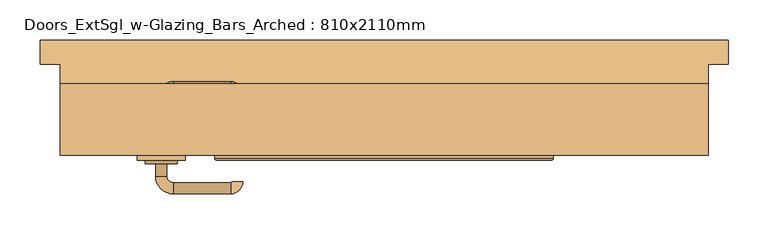
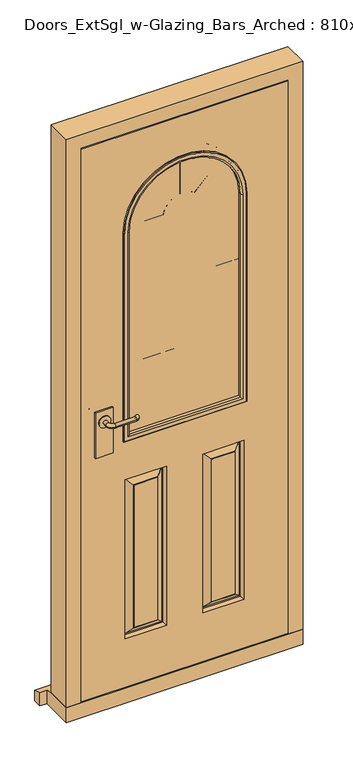
"""IFC4 building model written with IfcOpenShell, lengths in millimetres: door geometry, Doors_ExtSgl_w-Glazing_Bars_Arched : 810x2110mm."""

from ifc_helpers import new_model, si_unit, point, frame, frame_2d, origin, place, context, project, spatial, polyline, circle_curve, ellipse_curve, trimmed, segment, composite_curve, outline, extrude, faceted_brep, source, transform, mapped, element, save
from ifc_brep_helpers import plane_surface, cylinder_surface, revolved_surface, advanced_brep


def doors_extsgl_w_glazing_bars_arched_810x2110mm_57ea6d9e(model_context):
    return source(origin(), model_context, "Body", "SolidModel", [
        extrude(outline(composite_curve([segment(trimmed(circle_curve(frame_2d((1050.0, -278.5)), 20.0), [point((1050.0, -298.5))], [point((1050.0, -258.5))], False, "CARTESIAN"), True, "CONTINUOUS"), segment(trimmed(circle_curve(frame_2d((1050.0, -278.5)), 20.0), [point((1050.0, -258.5))], [point((1050.0, -298.5))], False, "CARTESIAN"), True, "CONTINUOUS")], self_intersect=False)), frame((0.0, -22.9929895, 0.0), z_axis=(0.0, 1.0, 0.0), x_axis=(0.0, 0.0, 1.0)), (0.0, 0.0, 1.0), 4.5929895),
        advanced_brep(
        [(-271.5, -22.9929895, 1050.0), (-285.5, -22.9929895, 1050.0), (-285.5, -38.4, 1050.0), (-271.5, -38.4, 1050.0), (-263.5, -60.4, 1050.0), (-263.5, -46.4, 1050.0), (-191.5, -60.4, 1050.0), (-191.5, -46.4, 1050.0), (-190.5, -45.4, 1050.0), (-176.5, -45.4, 1050.0)],
        [
            (0, 1, circle_curve(frame((-278.5, -22.9929895, 1050.0), z_axis=(0.0, 1.0, 0.0), x_axis=(-1.0, 0.0, 0.0)), 7.0)),
            (1, 0, circle_curve(frame((-278.5, -22.9929895, 1050.0), z_axis=(0.0, 1.0, 0.0), x_axis=(-1.0, 0.0, 0.0)), 7.0)),
            (1, 2),
            (2, 3, circle_curve(frame((-278.5, -38.4, 1050.0), z_axis=(0.0, 1.0, 0.0), x_axis=(-1.0, 0.0, 0.0)), 7.0)),
            (3, 0),
            (3, 2, circle_curve(frame((-278.5, -38.4, 1050.0), z_axis=(0.0, 1.0, 0.0), x_axis=(-1.0, 0.0, 0.0)), 7.0)),
            (4, 5, circle_curve(frame((-263.5, -53.4, 1050.0), z_axis=(-1.0, 0.0, 0.0), x_axis=(0.0, -1.0, 0.0)), 7.0)),
            (5, 3, circle_curve(frame((-263.5, -38.4, 1050.0), z_axis=(0.0, 0.0, -1.0), x_axis=(-1.0, 0.0, 0.0)), 8.0)),
            (2, 4, circle_curve(frame((-263.5, -38.4, 1050.0), z_axis=(0.0, 0.0, 1.0), x_axis=(-1.0, 0.0, 0.0)), 22.0)),
            (5, 4, circle_curve(frame((-263.5, -53.4, 1050.0), z_axis=(-1.0, 0.0, 0.0), x_axis=(0.0, -1.0, 0.0)), 7.0)),
            (4, 6),
            (6, 7, circle_curve(frame((-191.5, -53.4, 1050.0), z_axis=(-1.0, 0.0, 0.0), x_axis=(0.0, -1.0, 0.0)), 7.0)),
            (7, 5),
            (7, 6, circle_curve(frame((-191.5, -53.4, 1050.0), z_axis=(-1.0, 0.0, 0.0), x_axis=(0.0, -1.0, 0.0)), 7.0)),
            (8, 9, circle_curve(frame((-183.5, -45.4, 1050.0), z_axis=(0.0, 1.0, 0.0), x_axis=(1.0, 0.0, 0.0)), 7.0)),
            (9, 8, circle_curve(frame((-183.5, -45.4, 1050.0), z_axis=(0.0, 1.0, 0.0), x_axis=(1.0, 0.0, 0.0)), 7.0)),
            (8, 7, circle_curve(frame((-191.5, -45.4, 1050.0), z_axis=(0.0, 0.0, -1.0), x_axis=(0.0, -1.0, 0.0)), 1.0)),
            (6, 9, circle_curve(frame((-191.5, -45.4, 1050.0), z_axis=(0.0, 0.0, 1.0), x_axis=(0.0, -1.0, 0.0)), 15.0)),
        ],
        [
            plane_surface(frame((-278.5, -22.9929895, 1050.0), z_axis=(0.0, 1.0, 0.0), x_axis=(0.0, 0.0, 1.0))),
            cylinder_surface(frame((-278.5, -22.9929895, 1050.0), z_axis=(0.0, 1.0, 0.0), x_axis=(-1.0, 0.0, 0.0)), 7.0),
            revolved_surface(trimmed(ellipse_curve(frame((-278.5, -38.4, 1050.0), z_axis=(0.0, -1.0, 0.0), x_axis=(-1.0, 0.0, 0.0)), 7.0, 7.0), [point((-271.5, -38.4, 1050.0))], [point((-285.5, -38.4, 1050.0))], True, "CARTESIAN"), (-263.5, -38.4, 1050.0), (0.0, 0.0, -1.0)),
            revolved_surface(trimmed(ellipse_curve(frame((-278.5, -38.4, 1050.0), z_axis=(0.0, -1.0, 0.0), x_axis=(-1.0, 0.0, 0.0)), 7.0, 7.0), [point((-285.5, -38.4, 1050.0))], [point((-271.5, -38.4, 1050.0))], True, "CARTESIAN"), (-263.5, -38.4, 1050.0), (0.0, 0.0, -1.0)),
            cylinder_surface(frame((-263.5, -53.4, 1050.0), z_axis=(-1.0, 0.0, 0.0), x_axis=(0.0, -1.0, 0.0)), 7.0),
            plane_surface(frame((-183.5, -45.4, 1050.0), z_axis=(0.0, 1.0, 0.0), x_axis=(0.0, 0.0, 1.0))),
            revolved_surface(trimmed(ellipse_curve(frame((-191.5, -53.4, 1050.0), z_axis=(1.0, 0.0, 0.0), x_axis=(0.0, -1.0, 0.0)), 7.0, 7.0), [point((-191.5, -46.4, 1050.0))], [point((-191.5, -60.4, 1050.0))], True, "CARTESIAN"), (-191.5, -45.4, 1050.0), (0.0, 0.0, -1.0)),
            revolved_surface(trimmed(ellipse_curve(frame((-191.5, -53.4, 1050.0), z_axis=(1.0, 0.0, 0.0), x_axis=(0.0, -1.0, 0.0)), 7.0, 7.0), [point((-191.5, -60.4, 1050.0))], [point((-191.5, -46.4, 1050.0))], True, "CARTESIAN"), (-191.5, -45.4, 1050.0), (0.0, 0.0, -1.0)),
        ],
        [
            (0, [[1, 2]]),
            (1, [[3, 4, 5, -2]]),
            (1, [[-5, 6, -3, -1]]),
            (2, [[7, 8, -4, 9]]),
            (3, [[10, -9, -6, -8]]),
            (4, [[11, 12, 13, -7]]),
            (4, [[-13, 14, -11, -10]]),
            (5, [[15, 16]]),
            (6, [[-15, 17, -12, 18]]),
            (7, [[-16, -18, -14, -17]]),
        ],
    ),
        extrude(outline(polyline([(-248.5, -12.4), (-248.5, -18.4), (-308.5, -18.4), (-308.5, -12.4), (-248.5, -12.4)])), frame((0.0, 0.0, 925.0), z_axis=(0.0, 0.0, 1.0), x_axis=(1.0, 0.0, 0.0)), (0.0, 0.0, 1.0), 165.0),
        extrude(outline(composite_curve([segment(trimmed(circle_curve(frame_2d((1050.0, -278.5)), 20.0), [point((1050.0, -298.5))], [point((1050.0, -258.5))], False, "CARTESIAN"), True, "CONTINUOUS"), segment(trimmed(circle_curve(frame_2d((1050.0, -278.5)), 20.0), [point((1050.0, -258.5))], [point((1050.0, -298.5))], False, "CARTESIAN"), True, "CONTINUOUS")], self_intersect=False)), frame((0.0, 37.6, 0.0), z_axis=(0.0, 1.0, 0.0), x_axis=(0.0, 0.0, 1.0)), (0.0, 0.0, 1.0), 4.5929895),
        advanced_brep(
        [(-271.5, 42.1929895, 1050.0), (-285.5, 42.1929895, 1050.0), (-271.5, 57.6, 1050.0), (-285.5, 57.6, 1050.0), (-263.5, 79.6, 1050.0), (-263.5, 65.6, 1050.0), (-191.5, 65.6, 1050.0), (-191.5, 79.6, 1050.0), (-190.5, 64.6, 1050.0), (-176.5, 64.6, 1050.0)],
        [
            (0, 1, circle_curve(frame((-278.5, 42.1929895, 1050.0), z_axis=(0.0, -1.0, 0.0), x_axis=(-1.0, 0.0, 0.0)), 7.0)),
            (1, 0, circle_curve(frame((-278.5, 42.1929895, 1050.0), z_axis=(0.0, -1.0, 0.0), x_axis=(-1.0, 0.0, 0.0)), 7.0)),
            (0, 2),
            (2, 3, circle_curve(frame((-278.5, 57.6, 1050.0), z_axis=(0.0, -1.0, 0.0), x_axis=(-1.0, 0.0, 0.0)), 7.0)),
            (3, 1),
            (3, 2, circle_curve(frame((-278.5, 57.6, 1050.0), z_axis=(0.0, -1.0, 0.0), x_axis=(-1.0, 0.0, 0.0)), 7.0)),
            (4, 3, circle_curve(frame((-263.5, 57.6, 1050.0), z_axis=(0.0, 0.0, 1.0), x_axis=(-1.0, 0.0, 0.0)), 22.0)),
            (2, 5, circle_curve(frame((-263.5, 57.6, 1050.0), z_axis=(0.0, 0.0, -1.0), x_axis=(-1.0, 0.0, 0.0)), 8.0)),
            (5, 4, circle_curve(frame((-263.5, 72.6, 1050.0), z_axis=(-1.0, 0.0, 0.0), x_axis=(0.0, 1.0, 0.0)), 7.0)),
            (4, 5, circle_curve(frame((-263.5, 72.6, 1050.0), z_axis=(-1.0, 0.0, 0.0), x_axis=(0.0, 1.0, 0.0)), 7.0)),
            (5, 6),
            (6, 7, circle_curve(frame((-191.5, 72.6, 1050.0), z_axis=(-1.0, 0.0, 0.0), x_axis=(0.0, 1.0, 0.0)), 7.0)),
            (7, 4),
            (7, 6, circle_curve(frame((-191.5, 72.6, 1050.0), z_axis=(-1.0, 0.0, 0.0), x_axis=(0.0, 1.0, 0.0)), 7.0)),
            (8, 9, circle_curve(frame((-183.5, 64.6, 1050.0), z_axis=(0.0, -1.0, 0.0), x_axis=(1.0, 0.0, 0.0)), 7.0)),
            (9, 8, circle_curve(frame((-183.5, 64.6, 1050.0), z_axis=(0.0, -1.0, 0.0), x_axis=(1.0, 0.0, 0.0)), 7.0)),
            (9, 7, circle_curve(frame((-191.5, 64.6, 1050.0), z_axis=(0.0, 0.0, 1.0), x_axis=(0.0, 1.0, 0.0)), 15.0)),
            (6, 8, circle_curve(frame((-191.5, 64.6, 1050.0), z_axis=(0.0, 0.0, -1.0), x_axis=(0.0, 1.0, 0.0)), 1.0)),
        ],
        [
            plane_surface(frame((-278.5, 42.1929895, 1050.0), z_axis=(0.0, -1.0, 0.0), x_axis=(0.0, 0.0, 1.0))),
            cylinder_surface(frame((-278.5, 42.1929895, 1050.0), z_axis=(0.0, -1.0, 0.0), x_axis=(-1.0, 0.0, 0.0)), 7.0),
            revolved_surface(trimmed(ellipse_curve(frame((-278.5, 57.6, 1050.0), z_axis=(0.0, -1.0, 0.0), x_axis=(-1.0, 0.0, 0.0)), 7.0, 7.0), [point((-271.5, 57.6, 1050.0))], [point((-285.5, 57.6, 1050.0))], True, "CARTESIAN"), (-263.5, 57.6, 1050.0), (0.0, 0.0, -1.0)),
            revolved_surface(trimmed(ellipse_curve(frame((-278.5, 57.6, 1050.0), z_axis=(0.0, -1.0, 0.0), x_axis=(-1.0, 0.0, 0.0)), 7.0, 7.0), [point((-285.5, 57.6, 1050.0))], [point((-271.5, 57.6, 1050.0))], True, "CARTESIAN"), (-263.5, 57.6, 1050.0), (0.0, 0.0, -1.0)),
            cylinder_surface(frame((-263.5, 72.6, 1050.0), z_axis=(-1.0, 0.0, 0.0), x_axis=(0.0, 1.0, 0.0)), 7.0),
            plane_surface(frame((-183.5, 64.6, 1050.0), z_axis=(0.0, -1.0, 0.0), x_axis=(0.0, 0.0, 1.0))),
            revolved_surface(trimmed(ellipse_curve(frame((-191.5, 72.6, 1050.0), z_axis=(-1.0, 0.0, 0.0), x_axis=(0.0, 1.0, 0.0)), 7.0, 7.0), [point((-191.5, 65.6, 1050.0))], [point((-191.5, 79.6, 1050.0))], True, "CARTESIAN"), (-191.5, 64.6, 1050.0), (0.0, 0.0, -1.0)),
            revolved_surface(trimmed(ellipse_curve(frame((-191.5, 72.6, 1050.0), z_axis=(-1.0, 0.0, 0.0), x_axis=(0.0, 1.0, 0.0)), 7.0, 7.0), [point((-191.5, 79.6, 1050.0))], [point((-191.5, 65.6, 1050.0))], True, "CARTESIAN"), (-191.5, 64.6, 1050.0), (0.0, 0.0, -1.0)),
        ],
        [
            (0, [[1, 2]]),
            (1, [[-1, 3, 4, 5]]),
            (1, [[-2, -5, 6, -3]]),
            (2, [[7, -4, 8, 9]]),
            (3, [[-8, -6, -7, 10]]),
            (4, [[-9, 11, 12, 13]]),
            (4, [[-10, -13, 14, -11]]),
            (5, [[15, 16]]),
            (6, [[17, -12, 18, -16]]),
            (7, [[-18, -14, -17, -15]]),
        ],
    ),
        extrude(outline(polyline([(-248.5, 31.6), (-308.5, 31.6), (-308.5, 37.6), (-248.5, 37.6), (-248.5, 31.6)])), frame((0.0, 0.0, 925.0), z_axis=(0.0, 0.0, 1.0), x_axis=(1.0, 0.0, 0.0)), (0.0, 0.0, 1.0), 165.0),
        faceted_brep([(334.5, 76.6, 54.5), (405.0, 76.6, 54.5), (405.0, -12.4, 54.5), (356.5, -12.4, 54.5), (356.5, 34.6, 54.5), (334.5, 34.6, 54.5), (334.5, 76.6, 2039.5), (-334.5, 76.6, 2039.5), (-334.5, 76.6, 54.5), (-405.0, 76.6, 54.5), (-405.0, 76.6, 2110.0), (405.0, 76.6, 2110.0), (405.0, -12.4, 2110.0), (-405.0, -12.4, 2110.0), (-405.0, -12.4, 54.5), (-356.5, -12.4, 54.5), (-356.5, -12.4, 2061.5), (356.5, -12.4, 2061.5), (356.5, 34.6, 2061.5), (-356.5, 34.6, 2061.5), (-356.5, 34.6, 54.5), (-334.5, 34.6, 54.5), (-334.5, 34.6, 2039.5), (334.5, 34.6, 2039.5)], [[[0, 1, 2, 3, 4, 5]], [[1, 0, 6, 7, 8, 9, 10, 11]], [[2, 1, 11, 12]], [[3, 2, 12, 13, 14, 15, 16, 17]], [[4, 3, 17, 18]], [[5, 4, 18, 19, 20, 21, 22, 23]], [[0, 5, 23, 6]], [[8, 7, 22, 21]], [[9, 8, 21, 20, 15, 14]], [[10, 9, 14, 13]], [[16, 15, 20, 19]], [[11, 10, 13, 12]], [[17, 16, 19, 18]], [[7, 6, 23, 22]]]),
        advanced_brep(
        [(353.5, -12.4, 58.5), (353.5, -12.4, 2058.5), (-354.4250294, -12.4, 2058.5), (-354.4250294, -12.4, 58.5), (-203.5, -12.4, 958.5), (-203.5, -12.4, 1705.0), (203.5, -12.4, 1705.0), (203.5, -12.4, 958.5), (-62.5, -12.4, 808.5), (-62.5, -12.4, 233.5), (-203.5, -12.4, 233.5), (-203.5, -12.4, 808.5), (203.5, -12.4, 808.5), (203.5, -12.4, 233.5), (62.5, -12.4, 233.5), (62.5, -12.4, 808.5), (-92.5, -12.4, 263.5), (-92.5, -12.4, 778.5), (-173.5, -12.4, 778.5), (-173.5, -12.4, 263.5), (173.5, -12.4, 263.5), (173.5, -12.4, 778.5), (92.5, -12.4, 778.5), (92.5, -12.4, 263.5), (353.5, 31.6, 58.5), (-354.4250294, 31.6, 58.5), (-354.4250294, 31.6, 2058.5), (353.5, 31.6, 2058.5), (-203.5, 31.6, 958.5), (203.5, 31.6, 958.5), (203.5, 31.6, 1705.0), (-203.5, 31.6, 1705.0), (62.5, 31.6, 808.5), (62.5, 31.6, 233.5), (203.5, 31.6, 233.5), (203.5, 31.6, 808.5), (-203.5, 31.6, 808.5), (-203.5, 31.6, 233.5), (-62.5, 31.6, 233.5), (-62.5, 31.6, 808.5), (92.5, 31.6, 263.5), (92.5, 31.6, 778.5), (173.5, 31.6, 778.5), (173.5, 31.6, 263.5), (-173.5, 31.6, 263.5), (-173.5, 31.6, 778.5), (-92.5, 31.6, 778.5), (-92.5, 31.6, 263.5), (65.5, 16.6, 805.5), (65.5, 16.6, 236.5), (90.5, 30.6, 780.5), (90.5, 30.6, 261.5), (70.5, 16.6, 241.5), (70.5, 16.6, 800.5), (92.5, 30.6, 263.5), (92.5, 30.6, 778.5), (200.5, 16.6, 236.5), (175.5, 30.6, 261.5), (195.5, 16.6, 241.5), (173.5, 30.6, 263.5), (200.5, 16.6, 805.5), (175.5, 30.6, 780.5), (195.5, 16.6, 800.5), (173.5, 30.6, 778.5), (-200.5, 16.6, 805.5), (-200.5, 16.6, 236.5), (-175.5, 30.6, 780.5), (-175.5, 30.6, 261.5), (-195.5, 16.6, 241.5), (-195.5, 16.6, 800.5), (-173.5, 30.6, 263.5), (-173.5, 30.6, 778.5), (-65.5, 16.6, 236.5), (-90.5, 30.6, 261.5), (-70.5, 16.6, 241.5), (-92.5, 30.6, 263.5), (-65.5, 16.6, 805.5), (-90.5, 30.6, 780.5), (-70.5, 16.6, 800.5), (-92.5, 30.6, 778.5), (-92.5, -11.4, 263.5), (-92.5, -11.4, 778.5), (-70.5, 2.6, 241.5), (-70.5, 2.6, 800.5), (-90.5, -11.4, 780.5), (-90.5, -11.4, 261.5), (-65.5, 2.6, 805.5), (-65.5, 2.6, 236.5), (-173.5, -11.4, 778.5), (-195.5, 2.6, 800.5), (-175.5, -11.4, 780.5), (-200.5, 2.6, 805.5), (-173.5, -11.4, 263.5), (-195.5, 2.6, 241.5), (-175.5, -11.4, 261.5), (-200.5, 2.6, 236.5), (200.5, 2.6, 805.5), (200.5, 2.6, 236.5), (175.5, -11.4, 780.5), (175.5, -11.4, 261.5), (195.5, 2.6, 241.5), (195.5, 2.6, 800.5), (173.5, -11.4, 263.5), (173.5, -11.4, 778.5), (65.5, 2.6, 236.5), (90.5, -11.4, 261.5), (70.5, 2.6, 241.5), (92.5, -11.4, 263.5), (65.5, 2.6, 805.5), (90.5, -11.4, 780.5), (70.5, 2.6, 800.5), (92.5, -11.4, 778.5)],
        [
            (0, 1),
            (1, 2),
            (2, 3),
            (3, 0),
            (4, 5),
            (5, 6, circle_curve(frame((0.0, -12.4, 1705.0), z_axis=(0.0, 1.0, 0.0), x_axis=(1.0, 0.0, 0.0)), 203.5)),
            (6, 7),
            (7, 4),
            (8, 9),
            (9, 10),
            (10, 11),
            (11, 8),
            (12, 13),
            (13, 14),
            (14, 15),
            (15, 12),
            (16, 17),
            (17, 18),
            (18, 19),
            (19, 16),
            (20, 21),
            (21, 22),
            (22, 23),
            (23, 20),
            (24, 25),
            (25, 26),
            (26, 27),
            (27, 24),
            (28, 29),
            (29, 30),
            (30, 31, circle_curve(frame((0.0, 31.6, 1705.0), z_axis=(0.0, -1.0, 0.0), x_axis=(1.0, 0.0, 0.0)), 203.5)),
            (31, 28),
            (32, 33),
            (33, 34),
            (34, 35),
            (35, 32),
            (36, 37),
            (37, 38),
            (38, 39),
            (39, 36),
            (40, 41),
            (41, 42),
            (42, 43),
            (43, 40),
            (44, 45),
            (45, 46),
            (46, 47),
            (47, 44),
            (0, 24),
            (27, 1),
            (26, 2),
            (25, 3),
            (4, 28),
            (31, 5),
            (30, 6),
            (29, 7),
            (48, 49),
            (49, 33),
            (32, 48),
            (50, 51),
            (51, 52),
            (52, 53),
            (53, 50),
            (40, 54),
            (54, 55),
            (55, 41),
            (49, 56),
            (56, 34),
            (51, 57),
            (57, 58),
            (58, 52),
            (43, 59),
            (59, 54),
            (56, 60),
            (60, 35),
            (57, 61),
            (61, 62),
            (62, 58),
            (42, 63),
            (63, 59),
            (60, 48),
            (62, 53),
            (61, 50),
            (63, 55),
            (64, 65),
            (65, 37),
            (36, 64),
            (66, 67),
            (67, 68),
            (68, 69),
            (69, 66),
            (44, 70),
            (70, 71),
            (71, 45),
            (65, 72),
            (72, 38),
            (67, 73),
            (73, 74),
            (74, 68),
            (47, 75),
            (75, 70),
            (72, 76),
            (76, 39),
            (73, 77),
            (77, 78),
            (78, 74),
            (46, 79),
            (79, 75),
            (76, 64),
            (78, 69),
            (77, 66),
            (79, 71),
            (80, 81),
            (81, 17),
            (16, 80),
            (82, 83),
            (83, 84),
            (84, 85),
            (85, 82),
            (8, 86),
            (86, 87),
            (87, 9),
            (81, 88),
            (88, 18),
            (83, 89),
            (89, 90),
            (90, 84),
            (11, 91),
            (91, 86),
            (88, 92),
            (92, 19),
            (89, 93),
            (93, 94),
            (94, 90),
            (10, 95),
            (95, 91),
            (92, 80),
            (94, 85),
            (93, 82),
            (95, 87),
            (96, 97),
            (97, 13),
            (12, 96),
            (98, 99),
            (99, 100),
            (100, 101),
            (101, 98),
            (20, 102),
            (102, 103),
            (103, 21),
            (97, 104),
            (104, 14),
            (99, 105),
            (105, 106),
            (106, 100),
            (23, 107),
            (107, 102),
            (104, 108),
            (108, 15),
            (105, 109),
            (109, 110),
            (110, 106),
            (22, 111),
            (111, 107),
            (108, 96),
            (110, 101),
            (109, 98),
            (111, 103),
        ],
        [
            plane_surface(frame((353.5, -12.4, 58.5), z_axis=(0.0, -1.0, 0.0), x_axis=(0.0, 0.0, 1.0))),
            plane_surface(frame((353.5, 31.6, 58.5), z_axis=(0.0, 1.0, 0.0), x_axis=(0.0, 0.0, -1.0))),
            plane_surface(frame((353.5, -12.4, 58.5), z_axis=(1.0, 0.0, 0.0), x_axis=(0.0, 1.0, 0.0))),
            plane_surface(frame((353.5, -12.4, 2058.5), z_axis=(0.0, 0.0, 1.0), x_axis=(0.0, 1.0, 0.0))),
            plane_surface(frame((-354.4250294, -12.4, 2058.5), z_axis=(-1.0, 0.0, 0.0), x_axis=(0.0, 1.0, 0.0))),
            plane_surface(frame((-354.4250294, -12.4, 58.5), z_axis=(0.0, 0.0, -1.0), x_axis=(0.0, 1.0, 0.0))),
            plane_surface(frame((-203.5, -12.4, 958.5), z_axis=(1.0, 0.0, 0.0), x_axis=(0.0, 1.0, 0.0))),
            revolved_surface(polyline([(203.5, 31.6, 1705.0), (203.5, -12.4, 1705.0)]), (0.0, -12.4, 1705.0), (0.0, 1.0, 0.0)),
            plane_surface(frame((203.5, -12.4, 1705.0), z_axis=(-1.0, 0.0, 0.0), x_axis=(0.0, 1.0, 0.0))),
            plane_surface(frame((203.5, -12.4, 958.5), z_axis=(0.0, 0.0, 1.0), x_axis=(0.0, 1.0, 0.0))),
            plane_surface(frame((62.5, 31.6, 808.5), z_axis=(0.9805806756909202, 0.19611613513818407, 0.0), x_axis=(0.0, 0.0, -1.0))),
            plane_surface(frame((70.5, 16.6, 800.5), z_axis=(-0.5734623443633278, 0.8192319205190408, 0.0), x_axis=(0.0, 0.0, -1.0))),
            plane_surface(frame((92.5, 30.6, 778.5), z_axis=(-1.0, 0.0, 0.0), x_axis=(0.0, 0.0, -1.0))),
            plane_surface(frame((62.5, 31.6, 233.5), z_axis=(0.0, 0.19611613513818718, 0.9805806756909196), x_axis=(1.0, 0.0, 0.0))),
            plane_surface(frame((70.5, 16.6, 241.5), z_axis=(0.0, 0.8192319205190389, -0.5734623443633305), x_axis=(1.0, 0.0, 0.0))),
            plane_surface(frame((92.5, 30.6, 263.5), z_axis=(0.0, 0.0, -1.0), x_axis=(1.0, 0.0, 0.0))),
            plane_surface(frame((203.5, 31.6, 233.5), z_axis=(-0.9805806756909189, 0.19611613513819035, 0.0), x_axis=(0.0, 0.0, 1.0))),
            plane_surface(frame((195.5, 16.6, 241.5), z_axis=(0.5734623443633332, 0.819231920519037, 0.0), x_axis=(0.0, 0.0, 1.0))),
            plane_surface(frame((173.5, 30.6, 263.5), z_axis=(1.0, 0.0, 0.0), x_axis=(0.0, 0.0, 1.0))),
            plane_surface(frame((203.5, 31.6, 808.5), z_axis=(0.0, 0.19611613513818718, -0.9805806756909196), x_axis=(-1.0, 0.0, 0.0))),
            plane_surface(frame((200.5, 16.6, 805.5), z_axis=(0.0, 1.0, 0.0), x_axis=(-1.0, 0.0, 0.0))),
            plane_surface(frame((195.5, 16.6, 800.5), z_axis=(0.0, 0.8192319205190389, 0.5734623443633305), x_axis=(-1.0, 0.0, 0.0))),
            plane_surface(frame((175.5, 30.6, 780.5), z_axis=(0.0, 1.0, 0.0), x_axis=(-1.0, 0.0, 0.0))),
            plane_surface(frame((173.5, 30.6, 778.5), z_axis=(0.0, 0.0, 1.0), x_axis=(-1.0, 0.0, 0.0))),
            plane_surface(frame((-203.5, 31.6, 808.5), z_axis=(0.9805806756909202, 0.19611613513818407, 0.0), x_axis=(0.0, 0.0, -1.0))),
            plane_surface(frame((-195.5, 16.6, 800.5), z_axis=(-0.5734623443633278, 0.8192319205190408, 0.0), x_axis=(0.0, 0.0, -1.0))),
            plane_surface(frame((-173.5, 30.6, 778.5), z_axis=(-1.0, 0.0, 0.0), x_axis=(0.0, 0.0, -1.0))),
            plane_surface(frame((-203.5, 31.6, 233.5), z_axis=(0.0, 0.19611613513818724, 0.9805806756909196), x_axis=(1.0, 0.0, 0.0))),
            plane_surface(frame((-195.5, 16.6, 241.5), z_axis=(0.0, 0.819231920519039, -0.5734623443633305), x_axis=(1.0, 0.0, 0.0))),
            plane_surface(frame((-173.5, 30.6, 263.5), z_axis=(0.0, 0.0, -1.0), x_axis=(1.0, 0.0, 0.0))),
            plane_surface(frame((-62.5, 31.6, 233.5), z_axis=(-0.9805806756909189, 0.1961161351381904, 0.0), x_axis=(0.0, 0.0, 1.0))),
            plane_surface(frame((-70.5, 16.6, 241.5), z_axis=(0.5734623443633332, 0.8192319205190371, 0.0), x_axis=(0.0, 0.0, 1.0))),
            plane_surface(frame((-92.5, 30.6, 263.5), z_axis=(1.0, 0.0, 0.0), x_axis=(0.0, 0.0, 1.0))),
            plane_surface(frame((-62.5, 31.6, 808.5), z_axis=(0.0, 0.19611613513818724, -0.9805806756909196), x_axis=(-1.0, 0.0, 0.0))),
            plane_surface(frame((-65.5, 16.6, 805.5), z_axis=(0.0, 1.0, 0.0), x_axis=(-1.0, 0.0, 0.0))),
            plane_surface(frame((-70.5, 16.6, 800.5), z_axis=(0.0, 0.819231920519039, 0.5734623443633305), x_axis=(-1.0, 0.0, 0.0))),
            plane_surface(frame((-90.5, 30.6, 780.5), z_axis=(0.0, 1.0, 0.0), x_axis=(-1.0, 0.0, 0.0))),
            plane_surface(frame((-92.5, 30.6, 778.5), z_axis=(0.0, 0.0, 1.0), x_axis=(-1.0, 0.0, 0.0))),
            plane_surface(frame((-92.5, -12.4, 263.5), z_axis=(1.0, 0.0, 0.0), x_axis=(0.0, 0.0, 1.0))),
            plane_surface(frame((-90.5, -11.4, 261.5), z_axis=(0.5734623443633226, -0.8192319205190445, 0.0), x_axis=(0.0, 0.0, 1.0))),
            plane_surface(frame((-65.5, 2.6, 236.5), z_axis=(-0.9805806756909214, -0.1961161351381777, 0.0), x_axis=(0.0, 0.0, 1.0))),
            plane_surface(frame((-92.5, -12.4, 778.5), z_axis=(0.0, 0.0, 1.0), x_axis=(-1.0, 0.0, 0.0))),
            plane_surface(frame((-90.5, -11.4, 780.5), z_axis=(0.0, -0.8192319205190427, 0.5734623443633253), x_axis=(-1.0, 0.0, 0.0))),
            plane_surface(frame((-65.5, 2.6, 805.5), z_axis=(0.0, -0.19611613513818085, -0.9805806756909208), x_axis=(-1.0, 0.0, 0.0))),
            plane_surface(frame((-173.5, -12.4, 778.5), z_axis=(-1.0, 0.0, 0.0), x_axis=(0.0, 0.0, -1.0))),
            plane_surface(frame((-175.5, -11.4, 780.5), z_axis=(-0.5734623443633281, -0.8192319205190407, 0.0), x_axis=(0.0, 0.0, -1.0))),
            plane_surface(frame((-200.5, 2.6, 805.5), z_axis=(0.9805806756909202, -0.196116135138184, 0.0), x_axis=(0.0, 0.0, -1.0))),
            plane_surface(frame((-173.5, -12.4, 263.5), z_axis=(0.0, 0.0, -1.0), x_axis=(1.0, 0.0, 0.0))),
            plane_surface(frame((-173.5, -11.4, 263.5), z_axis=(0.0, -1.0, 0.0), x_axis=(1.0, 0.0, 0.0))),
            plane_surface(frame((-175.5, -11.4, 261.5), z_axis=(0.0, -0.8192319205190426, -0.5734623443633253), x_axis=(1.0, 0.0, 0.0))),
            plane_surface(frame((-195.5, 2.6, 241.5), z_axis=(0.0, -1.0, 0.0), x_axis=(1.0, 0.0, 0.0))),
            plane_surface(frame((-200.5, 2.6, 236.5), z_axis=(0.0, -0.19611613513818088, 0.9805806756909209), x_axis=(1.0, 0.0, 0.0))),
            plane_surface(frame((203.5, -12.4, 808.5), z_axis=(-0.9805806756909202, -0.19611613513818407, 0.0), x_axis=(0.0, 0.0, -1.0))),
            plane_surface(frame((195.5, 2.6, 800.5), z_axis=(0.5734623443633278, -0.8192319205190408, 0.0), x_axis=(0.0, 0.0, -1.0))),
            plane_surface(frame((173.5, -11.4, 778.5), z_axis=(1.0, 0.0, 0.0), x_axis=(0.0, 0.0, -1.0))),
            plane_surface(frame((203.5, -12.4, 233.5), z_axis=(0.0, -0.19611613513818724, 0.9805806756909196), x_axis=(-1.0, 0.0, 0.0))),
            plane_surface(frame((195.5, 2.6, 241.5), z_axis=(0.0, -0.819231920519039, -0.5734623443633305), x_axis=(-1.0, 0.0, 0.0))),
            plane_surface(frame((173.5, -11.4, 263.5), z_axis=(0.0, 0.0, -1.0), x_axis=(-1.0, 0.0, 0.0))),
            plane_surface(frame((62.5, -12.4, 233.5), z_axis=(0.9805806756909189, -0.19611613513819046, 0.0), x_axis=(0.0, 0.0, 1.0))),
            plane_surface(frame((70.5, 2.6, 241.5), z_axis=(-0.5734623443633331, -0.8192319205190371, 0.0), x_axis=(0.0, 0.0, 1.0))),
            plane_surface(frame((92.5, -11.4, 263.5), z_axis=(-1.0, 0.0, 0.0), x_axis=(0.0, 0.0, 1.0))),
            plane_surface(frame((62.5, -12.4, 808.5), z_axis=(0.0, -0.19611613513818724, -0.9805806756909196), x_axis=(1.0, 0.0, 0.0))),
            plane_surface(frame((65.5, 2.6, 805.5), z_axis=(0.0, -1.0, 0.0), x_axis=(1.0, 0.0, 0.0))),
            plane_surface(frame((70.5, 2.6, 800.5), z_axis=(0.0, -0.819231920519039, 0.5734623443633305), x_axis=(1.0, 0.0, 0.0))),
            plane_surface(frame((90.5, -11.4, 780.5), z_axis=(0.0, -1.0, 0.0), x_axis=(1.0, 0.0, 0.0))),
            plane_surface(frame((92.5, -11.4, 778.5), z_axis=(0.0, 0.0, 1.0), x_axis=(1.0, 0.0, 0.0))),
        ],
        [
            (0, [[1, 2, 3, 4], [5, 6, 7, 8], [9, 10, 11, 12], [13, 14, 15, 16]]),
            (0, [[17, 18, 19, 20]]),
            (0, [[21, 22, 23, 24]]),
            (1, [[25, 26, 27, 28], [29, 30, 31, 32], [33, 34, 35, 36], [37, 38, 39, 40]]),
            (1, [[41, 42, 43, 44]]),
            (1, [[45, 46, 47, 48]]),
            (2, [[-1, 49, -28, 50]]),
            (3, [[-2, -50, -27, 51]]),
            (4, [[-3, -51, -26, 52]]),
            (5, [[-4, -52, -25, -49]]),
            (6, [[-5, 53, -32, 54]]),
            (7, [[-6, -54, -31, 55]]),
            (8, [[-7, -55, -30, 56]]),
            (9, [[-8, -56, -29, -53]]),
            (10, [[57, 58, -33, 59]]),
            (11, [[60, 61, 62, 63]]),
            (12, [[64, 65, 66, -41]]),
            (13, [[-58, 67, 68, -34]]),
            (14, [[-61, 69, 70, 71]]),
            (15, [[-64, -44, 72, 73]]),
            (16, [[-68, 74, 75, -35]]),
            (17, [[-70, 76, 77, 78]]),
            (18, [[-72, -43, 79, 80]]),
            (19, [[-59, -36, -75, 81]]),
            (20, [[-57, -81, -74, -67], [-62, -71, -78, 82]]),
            (21, [[-63, -82, -77, 83]]),
            (22, [[-60, -83, -76, -69], [-65, -73, -80, 84]]),
            (23, [[-66, -84, -79, -42]]),
            (24, [[85, 86, -37, 87]]),
            (25, [[88, 89, 90, 91]]),
            (26, [[92, 93, 94, -45]]),
            (27, [[-86, 95, 96, -38]]),
            (28, [[-89, 97, 98, 99]]),
            (29, [[-92, -48, 100, 101]]),
            (30, [[-96, 102, 103, -39]]),
            (31, [[-98, 104, 105, 106]]),
            (32, [[-100, -47, 107, 108]]),
            (33, [[-87, -40, -103, 109]]),
            (34, [[-85, -109, -102, -95], [-90, -99, -106, 110]]),
            (35, [[-91, -110, -105, 111]]),
            (36, [[-88, -111, -104, -97], [-93, -101, -108, 112]]),
            (37, [[-94, -112, -107, -46]]),
            (38, [[113, 114, -17, 115]]),
            (39, [[116, 117, 118, 119]]),
            (40, [[120, 121, 122, -9]]),
            (41, [[-114, 123, 124, -18]]),
            (42, [[-117, 125, 126, 127]]),
            (43, [[-120, -12, 128, 129]]),
            (44, [[-124, 130, 131, -19]]),
            (45, [[-126, 132, 133, 134]]),
            (46, [[-128, -11, 135, 136]]),
            (47, [[-115, -20, -131, 137]]),
            (48, [[-118, -127, -134, 138], [-113, -137, -130, -123]]),
            (49, [[-119, -138, -133, 139]]),
            (50, [[-121, -129, -136, 140], [-116, -139, -132, -125]]),
            (51, [[-122, -140, -135, -10]]),
            (52, [[141, 142, -13, 143]]),
            (53, [[144, 145, 146, 147]]),
            (54, [[148, 149, 150, -21]]),
            (55, [[-142, 151, 152, -14]]),
            (56, [[-145, 153, 154, 155]]),
            (57, [[-148, -24, 156, 157]]),
            (58, [[-152, 158, 159, -15]]),
            (59, [[-154, 160, 161, 162]]),
            (60, [[-156, -23, 163, 164]]),
            (61, [[-143, -16, -159, 165]]),
            (62, [[-141, -165, -158, -151], [-146, -155, -162, 166]]),
            (63, [[-147, -166, -161, 167]]),
            (64, [[-144, -167, -160, -153], [-149, -157, -164, 168]]),
            (65, [[-150, -168, -163, -22]]),
        ],
    ),
        faceted_brep([(430.0, 131.6, 0.0), (430.0, 131.6, 38.5947221), (430.0, 101.6, 47.2703282), (430.0, 101.6, 0.0), (-430.0, 131.6, 38.5947221), (-430.0, 131.6, 0.0), (-430.0, 101.6, 0.0), (-430.0, 101.6, 47.2703282), (405.0, 101.6, 0.0), (405.0, -12.4, 0.0), (-405.0, -12.4, 0.0), (-405.0, 101.6, 0.0), (-405.0, 101.6, 47.2703282), (-405.0, 76.6, 54.5), (405.0, 76.6, 54.5), (405.0, 101.6, 47.2703282), (-405.0, -12.4, 54.5), (405.0, -12.4, 54.5)], [[[0, 1, 2, 3]], [[4, 5, 6, 7]], [[5, 0, 3, 8, 9, 10, 11, 6]], [[1, 0, 5, 4]], [[1, 4, 7, 12, 13, 14, 15, 2]], [[13, 16, 17, 14]], [[16, 10, 9, 17]], [[12, 11, 10, 16, 13]], [[11, 12, 7, 6]], [[8, 15, 14, 17, 9]], [[15, 8, 3, 2]]]),
        extrude(outline(composite_curve([segment(polyline([(958.5, -203.5), (958.5, 203.5), (1705.0, 203.5)]), True, "CONTINUOUS"), segment(trimmed(circle_curve(frame_2d((1705.0, 0.0)), 203.5), [point((1705.0, 203.5))], [point((1705.0, -203.5))], False, "CARTESIAN"), True, "CONTINUOUS"), segment(polyline([(1705.0, -203.5), (958.5, -203.5)]), True, "CONTINUOUS")], self_intersect=False)), frame((0.0, -2.4, 0.0), z_axis=(0.0, 1.0, 0.0), x_axis=(0.0, 0.0, 1.0)), (0.0, 0.0, 1.0), 24.0),
        advanced_brep(
        [(-211.5, 35.6, 950.5), (-211.5, 31.6, 950.5), (-211.5, 31.6, 1705.0), (-211.5, 35.6, 1705.0), (-209.5, 37.6, 952.5), (-209.5, 37.6, 1705.0), (-191.5, 32.6, 970.5), (-196.5, 37.6, 965.5), (-196.5, 37.6, 1705.0), (-191.5, 32.6, 1705.0), (-191.5, 21.6, 970.5), (-191.5, 21.6, 1705.0), (-203.5, 31.6, 958.5), (-203.5, 21.6, 958.5), (-203.5, 21.6, 1705.0), (-203.5, 31.6, 1705.0), (211.5, 35.6, 1705.0), (211.5, 31.6, 1705.0), (209.5, 37.6, 1705.0), (209.5, 37.6, 952.5), (196.5, 37.6, 1705.0), (196.5, 37.6, 965.5), (191.5, 32.6, 1705.0), (191.5, 21.6, 1705.0), (203.5, 21.6, 1705.0), (203.5, 21.6, 958.5), (191.5, 21.6, 970.5), (203.5, 31.6, 1705.0), (211.5, 31.6, 950.5), (203.5, 31.6, 958.5), (211.5, 35.6, 950.5), (191.5, 32.6, 970.5)],
        [
            (0, 1),
            (1, 2),
            (2, 3),
            (3, 0),
            (4, 0, ellipse_curve(frame((-209.5, 35.6, 952.5), z_axis=(-0.7071067811865475, 0.0, 0.7071067811865475), x_axis=(-0.7071067811865472, 0.0, -0.7071067811865477)), 2.8284271, 2.0)),
            (3, 5, circle_curve(frame((-209.5, 35.6, 1705.0), z_axis=(0.0, 0.0, -1.0), x_axis=(-1.0, 0.0, 0.0)), 2.0)),
            (5, 4),
            (6, 7, ellipse_curve(frame((-196.5, 32.6, 965.5), z_axis=(-0.7071067811865475, 0.0, 0.7071067811865475), x_axis=(-0.7071067811865472, 0.0, -0.7071067811865477)), 7.0710678, 5.0)),
            (7, 8),
            (8, 9, circle_curve(frame((-196.5, 32.6, 1705.0), z_axis=(0.0, 0.0, -1.0), x_axis=(-1.0, 0.0, 0.0)), 5.0)),
            (9, 6),
            (10, 6),
            (9, 11),
            (11, 10),
            (12, 13),
            (13, 14),
            (14, 15),
            (15, 12),
            (16, 3, circle_curve(frame((0.0, 35.6, 1705.0), z_axis=(0.0, -1.0, 0.0), x_axis=(-1.0, 0.0, 0.0)), 211.5)),
            (2, 17, circle_curve(frame((0.0, 31.6, 1705.0), z_axis=(0.0, 1.0, 0.0), x_axis=(-1.0, 0.0, 0.0)), 211.5)),
            (17, 16),
            (18, 5, circle_curve(frame((0.0, 37.6, 1705.0), z_axis=(0.0, -1.0, 0.0), x_axis=(-1.0, 0.0, 0.0)), 209.5)),
            (16, 18, circle_curve(frame((209.5, 35.6, 1705.0), z_axis=(0.0, 0.0, 1.0), x_axis=(1.0, 0.0, 0.0)), 2.0)),
            (18, 19),
            (19, 4),
            (20, 8, circle_curve(frame((0.0, 37.6, 1705.0), z_axis=(0.0, -1.0, 0.0), x_axis=(-1.0, 0.0, 0.0)), 196.5)),
            (7, 21),
            (21, 20),
            (22, 9, circle_curve(frame((0.0, 32.6, 1705.0), z_axis=(0.0, -1.0, 0.0), x_axis=(-1.0, 0.0, 0.0)), 191.5)),
            (20, 22, circle_curve(frame((196.5, 32.6, 1705.0), z_axis=(0.0, 0.0, 1.0), x_axis=(1.0, 0.0, 0.0)), 5.0)),
            (23, 11, circle_curve(frame((0.0, 21.6, 1705.0), z_axis=(0.0, -1.0, 0.0), x_axis=(-1.0, 0.0, 0.0)), 191.5)),
            (22, 23),
            (24, 14, circle_curve(frame((0.0, 21.6, 1705.0), z_axis=(0.0, -1.0, 0.0), x_axis=(-1.0, 0.0, 0.0)), 203.5)),
            (13, 25),
            (25, 24),
            (23, 26),
            (26, 10),
            (27, 15, circle_curve(frame((0.0, 31.6, 1705.0), z_axis=(0.0, -1.0, 0.0), x_axis=(-1.0, 0.0, 0.0)), 203.5)),
            (24, 27),
            (1, 28),
            (28, 17),
            (27, 29),
            (29, 12),
            (28, 30),
            (30, 16),
            (30, 19, ellipse_curve(frame((209.5, 35.6, 952.5), z_axis=(0.7071067811865475, 0.0, 0.7071067811865475), x_axis=(-0.7071067811865475, 0.0, 0.7071067811865476)), 2.8284271, 2.0)),
            (21, 31, ellipse_curve(frame((196.5, 32.6, 965.5), z_axis=(0.7071067811865475, 0.0, 0.7071067811865475), x_axis=(-0.7071067811865475, 0.0, 0.7071067811865476)), 7.0710678, 5.0)),
            (31, 22),
            (31, 26),
            (25, 29),
            (0, 30),
            (6, 31),
        ],
        [
            plane_surface(frame((-211.5, 31.6, 950.5), z_axis=(-1.0, 0.0, 0.0), x_axis=(0.0, 0.0, 1.0))),
            cylinder_surface(frame((-209.5, 35.6, 958.5), z_axis=(0.0, 0.0, -1.0), x_axis=(-1.0, 0.0, 0.0)), 2.0),
            cylinder_surface(frame((-196.5, 32.6, 958.5), z_axis=(0.0, 0.0, -1.0), x_axis=(-1.0, 0.0, 0.0)), 5.0),
            plane_surface(frame((-191.5, 32.6, 970.5), z_axis=(1.0, 0.0, 0.0), x_axis=(0.0, 0.0, 1.0))),
            plane_surface(frame((-203.5, 21.6, 958.5), z_axis=(-1.0, 0.0, 0.0), x_axis=(0.0, 0.0, 1.0))),
            cylinder_surface(frame((0.0, 31.6, 1705.0), z_axis=(0.0, 1.0, 0.0), x_axis=(-1.0, 0.0, 0.0)), 211.5),
            revolved_surface(trimmed(ellipse_curve(frame((-209.5, 35.6, 1705.0), z_axis=(0.0, 0.0, -1.0), x_axis=(-1.0, 0.0, 0.0)), 2.0, 2.0), [point((-211.5, 35.6, 1705.0))], [point((-209.5, 37.6, 1705.0))], True, "CARTESIAN"), (0.0, 31.6, 1705.0), (0.0, 1.0, 0.0)),
            plane_surface(frame((0.0, 37.6, 1705.0), z_axis=(0.0, 1.0, 0.0), x_axis=(-1.0, 0.0, 0.0))),
            revolved_surface(trimmed(ellipse_curve(frame((-196.5, 32.6, 1705.0), z_axis=(0.0, 0.0, -1.0), x_axis=(-1.0, 0.0, 0.0)), 5.0, 5.0), [point((-196.5, 37.6, 1705.0))], [point((-191.5, 32.6, 1705.0))], True, "CARTESIAN"), (0.0, 31.6, 1705.0), (0.0, 1.0, 0.0)),
            revolved_surface(polyline([(-191.5, 32.6, 1705.0), (-191.5, 21.6, 1705.0)]), (0.0, 31.6, 1705.0), (0.0, 1.0, 0.0)),
            plane_surface(frame((0.0, 21.6, 1705.0), z_axis=(0.0, -1.0, 0.0), x_axis=(-1.0, 0.0, 0.0))),
            cylinder_surface(frame((0.0, 31.6, 1705.0), z_axis=(0.0, 1.0, 0.0), x_axis=(-1.0, 0.0, 0.0)), 203.5),
            plane_surface(frame((0.0, 31.6, 1705.0), z_axis=(0.0, -1.0, 0.0), x_axis=(-1.0, 0.0, 0.0))),
            plane_surface(frame((211.5, 31.6, 1705.0), z_axis=(1.0, 0.0, 0.0), x_axis=(0.0, 0.0, -1.0))),
            cylinder_surface(frame((209.5, 35.6, 1705.0), z_axis=(0.0, 0.0, 1.0), x_axis=(1.0, 0.0, 0.0)), 2.0),
            cylinder_surface(frame((196.5, 32.6, 1705.0), z_axis=(0.0, 0.0, 1.0), x_axis=(1.0, 0.0, 0.0)), 5.0),
            plane_surface(frame((191.5, 32.6, 1705.0), z_axis=(-1.0, 0.0, 0.0), x_axis=(0.0, 0.0, -1.0))),
            plane_surface(frame((203.5, 21.6, 1705.0), z_axis=(1.0, 0.0, 0.0), x_axis=(0.0, 0.0, -1.0))),
            plane_surface(frame((211.5, 31.6, 950.5), z_axis=(0.0, 0.0, -1.0), x_axis=(-1.0, 0.0, 0.0))),
            cylinder_surface(frame((203.5, 35.6, 952.5), z_axis=(1.0, 0.0, 0.0), x_axis=(0.0, 0.0, -1.0)), 2.0),
            cylinder_surface(frame((203.5, 32.6, 965.5), z_axis=(1.0, 0.0, 0.0), x_axis=(0.0, 0.0, -1.0)), 5.0),
            plane_surface(frame((191.5, 32.6, 970.5), z_axis=(0.0, 0.0, 1.0), x_axis=(-1.0, 0.0, 0.0))),
            plane_surface(frame((203.5, 21.6, 958.5), z_axis=(0.0, 0.0, -1.0), x_axis=(-1.0, 0.0, 0.0))),
        ],
        [
            (0, [[1, 2, 3, 4]]),
            (1, [[5, -4, 6, 7]]),
            (2, [[8, 9, 10, 11]]),
            (3, [[12, -11, 13, 14]]),
            (4, [[15, 16, 17, 18]]),
            (5, [[19, -3, 20, 21]]),
            (6, [[22, -6, -19, 23]]),
            (7, [[24, 25, -7, -22], [26, -9, 27, 28]]),
            (8, [[29, -10, -26, 30]]),
            (9, [[31, -13, -29, 32]]),
            (10, [[33, -16, 34, 35], [36, 37, -14, -31]]),
            (11, [[38, -17, -33, 39]]),
            (12, [[-20, -2, 40, 41], [42, 43, -18, -38]]),
            (13, [[-21, -41, 44, 45]]),
            (14, [[-23, -45, 46, -24]]),
            (15, [[-30, -28, 47, 48]]),
            (16, [[-32, -48, 49, -36]]),
            (17, [[-39, -35, 50, -42]]),
            (18, [[-44, -40, -1, 51]]),
            (19, [[-46, -51, -5, -25]]),
            (20, [[-47, -27, -8, 52]]),
            (21, [[-49, -52, -12, -37]]),
            (22, [[-50, -34, -15, -43]]),
        ],
    ),
        advanced_brep(
        [(211.5, -16.4, 950.5), (211.5, -12.4, 950.5), (211.5, -12.4, 1705.0), (211.5, -16.4, 1705.0), (209.5, -18.4, 952.5), (209.5, -18.4, 1705.0), (191.5, -13.4, 970.5), (196.5, -18.4, 965.5), (196.5, -18.4, 1705.0), (191.5, -13.4, 1705.0), (191.5, -2.4, 970.5), (191.5, -2.4, 1705.0), (203.5, -12.4, 958.5), (203.5, -2.4, 958.5), (203.5, -2.4, 1705.0), (203.5, -12.4, 1705.0), (-211.5, -16.4, 1705.0), (-211.5, -12.4, 1705.0), (-209.5, -18.4, 1705.0), (-209.5, -18.4, 952.5), (-196.5, -18.4, 1705.0), (-196.5, -18.4, 965.5), (-191.5, -13.4, 1705.0), (-191.5, -2.4, 1705.0), (-203.5, -2.4, 1705.0), (-203.5, -2.4, 958.5), (-191.5, -2.4, 970.5), (-203.5, -12.4, 1705.0), (-211.5, -12.4, 950.5), (-203.5, -12.4, 958.5), (-211.5, -16.4, 950.5), (-191.5, -13.4, 970.5)],
        [
            (0, 1),
            (1, 2),
            (2, 3),
            (3, 0),
            (4, 0, ellipse_curve(frame((209.5, -16.4, 952.5), z_axis=(0.7071067811865429, 0.0, 0.707106781186552), x_axis=(0.7071067811865519, 0.0, -0.707106781186543)), 2.8284271, 2.0)),
            (3, 5, circle_curve(frame((209.5, -16.4, 1705.0), z_axis=(0.0, 0.0, -1.0), x_axis=(1.0, 0.0, 0.0)), 2.0)),
            (5, 4),
            (6, 7, ellipse_curve(frame((196.5, -13.4, 965.5), z_axis=(0.7071067811865429, 0.0, 0.707106781186552), x_axis=(0.7071067811865519, 0.0, -0.707106781186543)), 7.0710678, 5.0)),
            (7, 8),
            (8, 9, circle_curve(frame((196.5, -13.4, 1705.0), z_axis=(0.0, 0.0, -1.0), x_axis=(1.0, 0.0, 0.0)), 5.0)),
            (9, 6),
            (10, 6),
            (9, 11),
            (11, 10),
            (12, 13),
            (13, 14),
            (14, 15),
            (15, 12),
            (16, 3, circle_curve(frame((0.0, -16.4, 1705.0), z_axis=(0.0, 1.0, 0.0), x_axis=(1.0, 0.0, 0.0)), 211.5)),
            (2, 17, circle_curve(frame((0.0, -12.4, 1705.0), z_axis=(0.0, -1.0, 0.0), x_axis=(1.0, 0.0, 0.0)), 211.5)),
            (17, 16),
            (18, 5, circle_curve(frame((0.0, -18.4, 1705.0), z_axis=(0.0, 1.0, 0.0), x_axis=(1.0, 0.0, 0.0)), 209.5)),
            (16, 18, circle_curve(frame((-209.5, -16.4, 1705.0), z_axis=(0.0, 0.0, 1.0), x_axis=(-1.0, 0.0, 0.0)), 2.0)),
            (18, 19),
            (19, 4),
            (20, 8, circle_curve(frame((0.0, -18.4, 1705.0), z_axis=(0.0, 1.0, 0.0), x_axis=(1.0, 0.0, 0.0)), 196.5)),
            (7, 21),
            (21, 20),
            (22, 9, circle_curve(frame((0.0, -13.4, 1705.0), z_axis=(0.0, 1.0, 0.0), x_axis=(1.0, 0.0, 0.0)), 191.5)),
            (20, 22, circle_curve(frame((-196.5, -13.4, 1705.0), z_axis=(0.0, 0.0, 1.0), x_axis=(-1.0, 0.0, 0.0)), 5.0)),
            (23, 11, circle_curve(frame((0.0, -2.4, 1705.0), z_axis=(0.0, 1.0, 0.0), x_axis=(1.0, 0.0, 0.0)), 191.5)),
            (22, 23),
            (24, 14, circle_curve(frame((0.0, -2.4, 1705.0), z_axis=(0.0, 1.0, 0.0), x_axis=(1.0, 0.0, 0.0)), 203.5)),
            (13, 25),
            (25, 24),
            (23, 26),
            (26, 10),
            (27, 15, circle_curve(frame((0.0, -12.4, 1705.0), z_axis=(0.0, 1.0, 0.0), x_axis=(1.0, 0.0, 0.0)), 203.5)),
            (24, 27),
            (1, 28),
            (28, 17),
            (27, 29),
            (29, 12),
            (28, 30),
            (30, 16),
            (30, 19, ellipse_curve(frame((-209.5, -16.4, 952.5), z_axis=(-0.707106781186552, 0.0, 0.7071067811865429), x_axis=(0.7071067811865428, 0.0, 0.7071067811865521)), 2.8284271, 2.0)),
            (21, 31, ellipse_curve(frame((-196.5, -13.4, 965.5), z_axis=(-0.707106781186552, 0.0, 0.7071067811865429), x_axis=(0.7071067811865428, 0.0, 0.7071067811865521)), 7.0710678, 5.0)),
            (31, 22),
            (31, 26),
            (25, 29),
            (0, 30),
            (6, 31),
        ],
        [
            plane_surface(frame((211.5, -12.4, 950.5), z_axis=(1.0, 0.0, 0.0), x_axis=(0.0, 0.0, 1.0))),
            cylinder_surface(frame((209.5, -16.4, 958.5), z_axis=(0.0, 0.0, -1.0), x_axis=(1.0, 0.0, 0.0)), 2.0),
            cylinder_surface(frame((196.5, -13.4, 958.5), z_axis=(0.0, 0.0, -1.0), x_axis=(1.0, 0.0, 0.0)), 5.0),
            plane_surface(frame((191.5, -13.4, 970.5), z_axis=(-1.0, 0.0, 0.0), x_axis=(0.0, 0.0, 1.0))),
            plane_surface(frame((203.5, -2.4, 958.5), z_axis=(1.0, 0.0, 0.0), x_axis=(0.0, 0.0, 1.0))),
            cylinder_surface(frame((0.0, -12.4, 1705.0), z_axis=(0.0, -1.0, 0.0), x_axis=(1.0, 0.0, 0.0)), 211.5),
            revolved_surface(trimmed(ellipse_curve(frame((209.5, -16.4, 1705.0), z_axis=(0.0, 0.0, -1.0), x_axis=(1.0, 0.0, 0.0)), 2.0, 2.0), [point((211.5, -16.4, 1705.0))], [point((209.5, -18.4, 1705.0))], True, "CARTESIAN"), (0.0, -12.4, 1705.0), (0.0, -1.0, 0.0)),
            plane_surface(frame((0.0, -18.4, 1705.0), z_axis=(0.0, -1.0, 0.0), x_axis=(1.0, 0.0, 0.0))),
            revolved_surface(trimmed(ellipse_curve(frame((196.5, -13.4, 1705.0), z_axis=(0.0, 0.0, -1.0), x_axis=(1.0, 0.0, 0.0)), 5.0, 5.0), [point((196.5, -18.4, 1705.0))], [point((191.5, -13.4, 1705.0))], True, "CARTESIAN"), (0.0, -12.4, 1705.0), (0.0, -1.0, 0.0)),
            revolved_surface(polyline([(191.5, -13.4, 1705.0), (191.5, -2.4000000000000004, 1705.0)]), (0.0, -12.4, 1705.0), (0.0, -1.0, 0.0)),
            plane_surface(frame((0.0, -2.4, 1705.0), z_axis=(0.0, 1.0, 0.0), x_axis=(1.0, 0.0, 0.0))),
            cylinder_surface(frame((0.0, -12.4, 1705.0), z_axis=(0.0, -1.0, 0.0), x_axis=(1.0, 0.0, 0.0)), 203.5),
            plane_surface(frame((0.0, -12.4, 1705.0), z_axis=(0.0, 1.0, 0.0), x_axis=(1.0, 0.0, 0.0))),
            plane_surface(frame((-211.5, -12.4, 1705.0), z_axis=(-1.0, 0.0, 0.0), x_axis=(0.0, 0.0, -1.0))),
            cylinder_surface(frame((-209.5, -16.4, 1705.0), z_axis=(0.0, 0.0, 1.0), x_axis=(-1.0, 0.0, 0.0)), 2.0),
            cylinder_surface(frame((-196.5, -13.4, 1705.0), z_axis=(0.0, 0.0, 1.0), x_axis=(-1.0, 0.0, 0.0)), 5.0),
            plane_surface(frame((-191.5, -13.4, 1705.0), z_axis=(1.0, 0.0, 0.0), x_axis=(0.0, 0.0, -1.0))),
            plane_surface(frame((-203.5, -2.4, 1705.0), z_axis=(-1.0, 0.0, 0.0), x_axis=(0.0, 0.0, -1.0))),
            plane_surface(frame((-211.5, -12.4, 950.5), z_axis=(0.0, 0.0, -1.0), x_axis=(1.0, 0.0, 0.0))),
            cylinder_surface(frame((-203.5, -16.4, 952.5), z_axis=(-1.0, 0.0, 0.0), x_axis=(0.0, 0.0, -1.0)), 2.0),
            cylinder_surface(frame((-203.5, -13.4, 965.5), z_axis=(-1.0, 0.0, 0.0), x_axis=(0.0, 0.0, -1.0)), 5.0),
            plane_surface(frame((-191.5, -13.4, 970.5), z_axis=(0.0, 0.0, 1.0), x_axis=(1.0, 0.0, 0.0))),
            plane_surface(frame((-203.5, -2.4, 958.5), z_axis=(0.0, 0.0, -1.0), x_axis=(1.0, 0.0, 0.0))),
        ],
        [
            (0, [[1, 2, 3, 4]]),
            (1, [[5, -4, 6, 7]]),
            (2, [[8, 9, 10, 11]]),
            (3, [[12, -11, 13, 14]]),
            (4, [[15, 16, 17, 18]]),
            (5, [[19, -3, 20, 21]]),
            (6, [[22, -6, -19, 23]]),
            (7, [[24, 25, -7, -22], [26, -9, 27, 28]]),
            (8, [[29, -10, -26, 30]]),
            (9, [[31, -13, -29, 32]]),
            (10, [[33, -16, 34, 35], [36, 37, -14, -31]]),
            (11, [[38, -17, -33, 39]]),
            (12, [[-20, -2, 40, 41], [42, 43, -18, -38]]),
            (13, [[-21, -41, 44, 45]]),
            (14, [[-23, -45, 46, -24]]),
            (15, [[-30, -28, 47, 48]]),
            (16, [[-32, -48, 49, -36]]),
            (17, [[-39, -35, 50, -42]]),
            (18, [[-44, -40, -1, 51]]),
            (19, [[-46, -51, -5, -25]]),
            (20, [[-47, -27, -8, 52]]),
            (21, [[-49, -52, -12, -37]]),
            (22, [[-50, -34, -15, -43]]),
        ],
    ),
        extrude(outline(composite_curve([segment(polyline([(958.5, 57.8333333), (958.5, 77.8333333), (1197.3333333, 77.8333333), (1197.3333333, 203.5), (1217.3333333, 203.5), (1217.3333333, 77.8333333), (1446.1666667, 77.8333333), (1446.1666667, 203.5), (1466.1666667, 203.5), (1466.1666667, 77.8333333), (1695.0, 77.8333333), (1695.0, 203.5), (1715.0, 203.5), (1715.0, 67.8333333)]), True, "CONTINUOUS"), segment(trimmed(circle_curve(frame_2d((1702.0, 0.0)), 69.0678008), [point((1715.0, 67.8333333))], [point((1744.9484515, 54.0905872))], False, "CARTESIAN"), True, "CONTINUOUS"), segment(polyline([(1744.9484515, 54.0905872), (1841.6513208, 150.7934565)]), True, "CONTINUOUS"), segment(trimmed(circle_curve(frame_2d((1705.0, 0.0)), 203.5), [point((1841.6513208, 150.7934565))], [point((1855.7934565, 136.6513208))], False, "CARTESIAN"), True, "CONTINUOUS"), segment(polyline([(1855.7934565, 136.6513208), (1758.6513897, 39.5092541)]), True, "CONTINUOUS"), segment(trimmed(circle_curve(frame_2d((1702.0, 0.0)), 69.0678008), [point((1758.6513897, 39.5092541))], [point((1770.3400403, 10.0))], False, "CARTESIAN"), True, "CONTINUOUS"), segment(polyline([(1770.3400403, 10.0), (1908.2541512, 10.0)]), True, "CONTINUOUS"), segment(trimmed(circle_curve(frame_2d((1705.0, 0.0)), 203.5), [point((1908.2541512, 10.0))], [point((1908.2541512, -10.0))], False, "CARTESIAN"), True, "CONTINUOUS"), segment(polyline([(1908.2541512, -10.0), (1770.3400403, -10.0)]), True, "CONTINUOUS"), segment(trimmed(circle_curve(frame_2d((1702.0, 0.0)), 69.0678008), [point((1770.3400403, -10.0))], [point((1758.6513897, -39.5092541))], False, "CARTESIAN"), True, "CONTINUOUS"), segment(polyline([(1758.6513897, -39.5092541), (1855.7934565, -136.6513208)]), True, "CONTINUOUS"), segment(trimmed(circle_curve(frame_2d((1705.0, 0.0)), 203.5), [point((1855.7934565, -136.6513208))], [point((1841.6513208, -150.7934565))], False, "CARTESIAN"), True, "CONTINUOUS"), segment(polyline([(1841.6513208, -150.7934565), (1744.9484515, -54.0905872)]), True, "CONTINUOUS"), segment(trimmed(circle_curve(frame_2d((1702.0, 0.0)), 69.0678008), [point((1744.9484515, -54.0905872))], [point((1715.0, -67.8333333))], False, "CARTESIAN"), True, "CONTINUOUS"), segment(polyline([(1715.0, -67.8333333), (1715.0, -203.5), (1695.0, -203.5), (1695.0, -77.8333333), (1466.1666667, -77.8333333), (1466.1666667, -203.5), (1446.1666667, -203.5), (1446.1666667, -77.8333333), (1217.3333333, -77.8333333), (1217.3333333, -203.5), (1197.3333333, -203.5), (1197.3333333, -77.8333333), (958.5, -77.8333333), (958.5, -57.8333333), (1197.3333333, -57.8333333), (1197.3333333, 57.8333333), (958.5, 57.8333333)]), True, "CONTINUOUS")], self_intersect=False), holes=[polyline([(1695.0, 57.8333333), (1466.1666667, 57.8333333), (1466.1666667, -57.8333333), (1695.0, -57.8333333), (1695.0, 57.8333333)]), polyline([(1446.1666667, -57.8333333), (1446.1666667, 57.8333333), (1217.3333333, 57.8333333), (1217.3333333, -57.8333333), (1446.1666667, -57.8333333)])]), frame((0.0, -2.4, 0.0), z_axis=(0.0, 1.0, 0.0), x_axis=(0.0, 0.0, 1.0)), (0.0, 0.0, 1.0), 24.0),
    ])


if __name__ == "__main__":
    model = new_model("IFC4")
    model_context = context("Model", 3, world=origin())
    ifc_project = project(units=[si_unit("LENGTHUNIT", "METRE", prefix="MILLI")], contexts=[model_context])
    site = spatial("IfcSite", under=ifc_project)
    building = spatial("IfcBuilding", under=site)
    placement = place(None, origin())
    doors_extsgl_w_glazing_bars_arched_810x2110mm_shape = doors_extsgl_w_glazing_bars_arched_810x2110mm_57ea6d9e(model_context)
    element("IfcDoor", 1, ObjectType="Doors_ExtSgl_w-Glazing_Bars_Arched : 810x2110mm", at=placement, inside=building, context=model_context, shape_type="MappedRepresentation", body=[
        mapped(doors_extsgl_w_glazing_bars_arched_810x2110mm_shape, transform((0.0, 0.0, 0.0), x_axis=(1.0, 0.0, 0.0), y_axis=(0.0, 1.0, 0.0), z_axis=(0.0, 0.0, 1.0))),
    ])
    save(model, "model.ifc")

# Revit data of these elements
# Type "Doors_ExtSgl_w-Glazing_Bars_Arched : 810x2110mm"
#   Type Mark = "9"
#   Type Comments = "External Single"
#   Operation = "SingleSwingRight"
#   Construction Type Id = "SGL"
#   Keynote = "L20"
#   Analytic Construction = "Large single-glazed windows"
#   Wrap Layers (Int) from Ext = 177.5 mm
#   Wrap Layers (Ext) from Ext = 102.5 mm
#   Visual Light Transmittance = 0.9
#   Thickness = 44 mm
#   Solar Heat Gain Coefficient = 0.86
#   Rough Width = 810 mm
#   Rough Height = 2110 mm
#   O/A Frame Width = 64 mm
#   Heat Transfer Coefficient (U) = 0.979472 BTU/(h·ft²·°F)
#   Handle Z Distance = 1050 mm
#   Glazing Thickness = 24 mm
#   FrameWidth = 42 mm
#   FrameOffset - External = 25 mm
#   FrameDepth = 89 mm
#   Door Panel Width = 707 mm
#   Door Panel Thickness = 44 mm
#   Door Panel Height = 2000 mm
#   DONT CHANGE - Half Glazed Width = 203.5 mm
#   DONT CHANGE - Glazed Width = 407 mm
#   Cill Thickness = 54.5 mm
#   Cill Projection = 30 mm
#   Handle X Distance = 75 mm
#   Height = 2110 mm
#   Structural Tolerance = 6.5 mm
#   Tolerance = 3 mm
#   Undercut = 4 mm
#   Width = 810 mm
#   Cill Extension = 25 mm
#   Cavity Closer Width = 50 mm
#   Cavity Closer Offset from Ext = 102.5 mm
#   Cavity Closer Depth = 85 mm
#   Vis - Ironmongery = yes
#   Vis - Glazing Bars = yes
#   Vis - Cavity Closers = yes
#   Define Thermal Properties by = 1
#   Function = 1
#   Material Glass = Door - Glazing
#   Material Glazing Bar = Door - Panel
#   Material Door = Door - Panel
#   Material Frame = Door - Frame/Mullion
#   Material Ironmongery = Door - Handle
#   Wall Closure = (empty or 0)
# Element 1 (IfcDoor, "Doors_ExtSgl_w-Glazing_Bars_Arched : 810x2110mm")
#   Materials on its faces: "Door - Panel", "Door - Handle", "Door - Frame/Mullion", "Door - Glazing"
# Materials
#   "Door - Glazing": colour RGB 0 0 255, transparency 0.75
#   "Door - Panel": class "Wood", colour RGB 210 159 95, transparency 0, Cost = 0
#   "Door - Frame/Mullion": class "Wood", colour RGB 212 179 113, transparency 0
#   "Door - Handle": colour RGB 246 240 166, transparency 0
